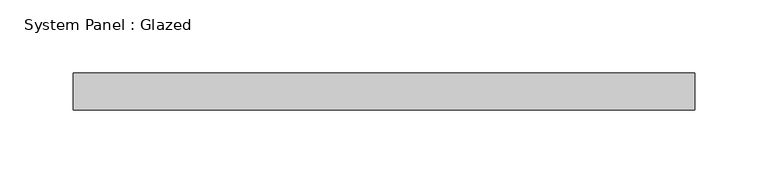
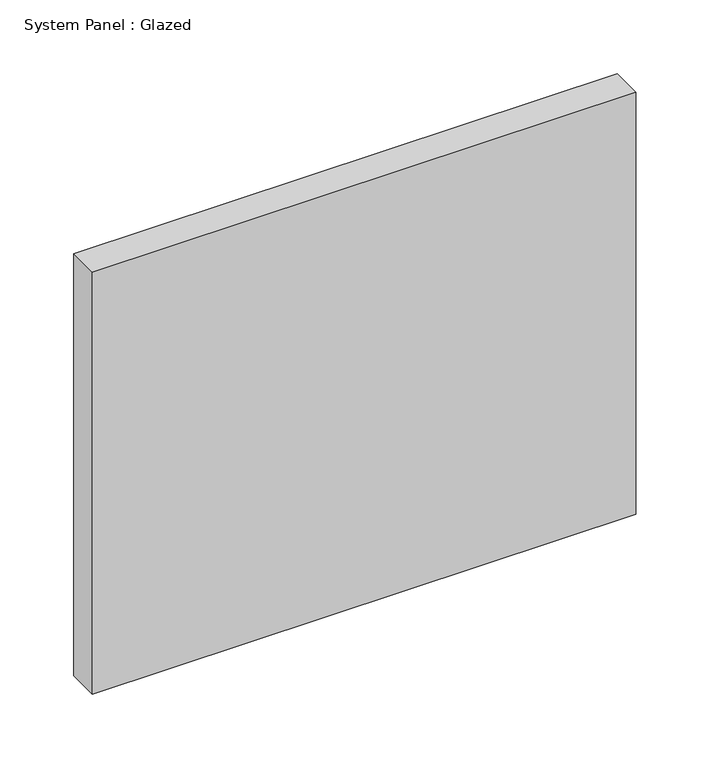
"""IFC4 building model written with IfcOpenShell, lengths in millimetres: plate geometry, System Panel : Glazed."""

from ifc_helpers import new_model, si_unit, origin, origin_with_axes, place, context, project, spatial, polyline, outline, extrude, source, transform, mapped, element, save


def system_panel_glazed_d5759347(model_context):
    return source(origin(), model_context, "Body", "SweptSolid", [
        extrude(outline(polyline([(212.725, 19.05), (-212.725, 19.05), (-212.725, 44.45), (212.725, 44.45), (212.725, 19.05)])), origin_with_axes(), (0.0, 0.0, 1.0), 349.25),
    ])


if __name__ == "__main__":
    model = new_model("IFC4")
    model_context = context("Model", 3, world=origin())
    ifc_project = project(units=[si_unit("LENGTHUNIT", "METRE", prefix="MILLI")], contexts=[model_context])
    site = spatial("IfcSite", under=ifc_project)
    building = spatial("IfcBuilding", under=site)
    placement = place(None, origin())
    system_panel_glazed_shape = system_panel_glazed_d5759347(model_context)
    element("IfcPlate", 1, ObjectType="System Panel : Glazed", at=placement, inside=building, context=model_context, shape_type="MappedRepresentation", body=[
        mapped(system_panel_glazed_shape, transform((0.0, 0.0, 0.0), x_axis=(1.0, 0.0, 0.0), y_axis=(0.0, 1.0, 0.0), z_axis=(0.0, 0.0, 1.0))),
    ])
    save(model, "model.ifc")

# Revit data of these elements
# Type "System Panel : Glazed"
#   Construction Type Id = "GSP4R"
#   Analytic Construction = "1/8 in Pilkington single glazing"
#   Visual Light Transmittance = 0.9
#   Solar Heat Gain Coefficient = 0.86
#   Heat Transfer Coefficient (U) = 1.18115 BTU/(h·ft²·°F)
#   Define Thermal Properties by = 1
# Element 1 (IfcPlate, "System Panel : Glazed")
#   Materials on its faces: "Glass"
# Materials
#   "Glass": class "Glass", colour RGB 0 128 192, transparency 0.75, Description = "Soda Lime Glass", Cost = 0
